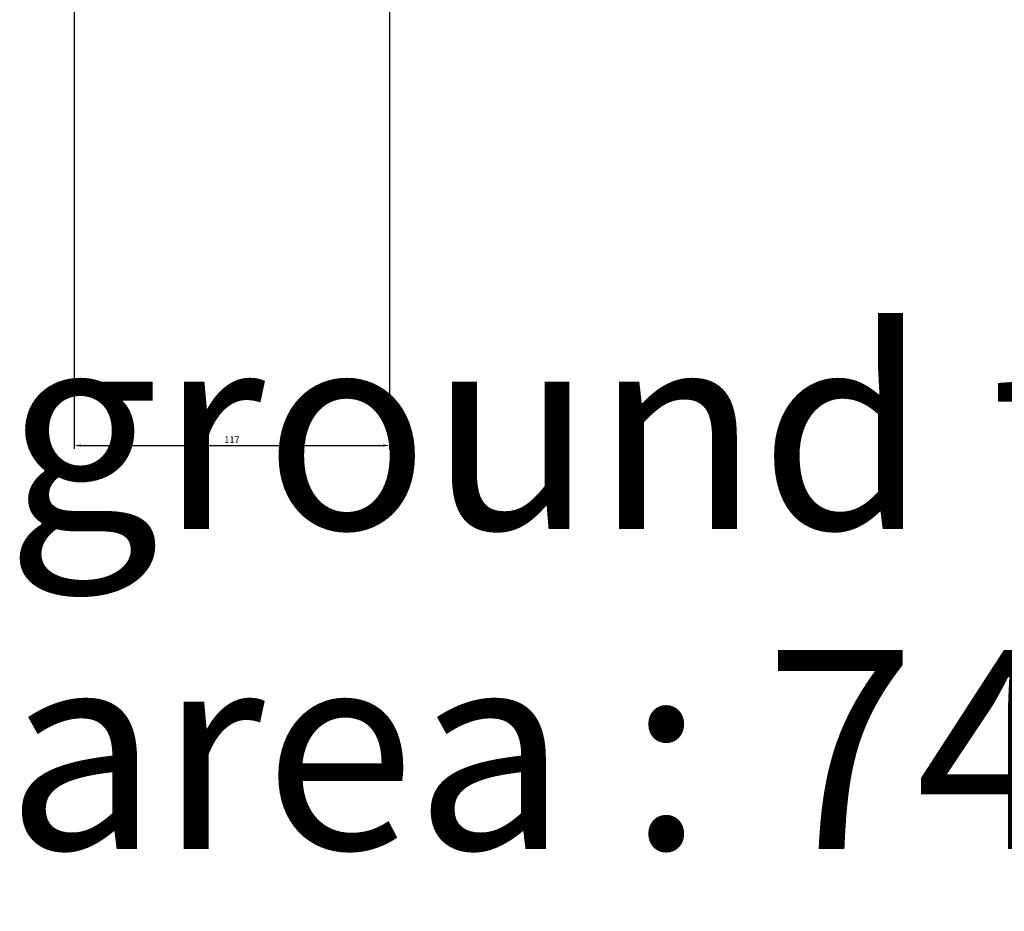
# Model space of a CAD drawing. Units: inches. Extents: x 604 to 3492, y -123 to 1737.
# Tile 1 of 20: x 673 to 1038, y -104 to 227. Entities that reach past the tile are written whole.
import ezdxf

# ---------------------------------------------------------------- set-up
doc = ezdxf.new("R2010")
doc.units = ezdxf.units.IN
for name, color, linetype, lineweight in [('A-ANNO-DIMS', 2, 'Continuous', 18), ('A-ANNO-TEXT', 7, 'Continuous', 35), ('A-AREA-IDEN', 7, 'Continuous', 25)]:
    doc.layers.add(name, color=color, linetype=linetype, lineweight=lineweight)
doc.styles.get("Standard").update_dxf_attribs({"font": 'arial.ttf'})
doc.dimstyles.new('ISO-25', dxfattribs={"dimtxt": 2.5, "dimasz": 2.5, "dimexe": 1.25, "dimexo": 0.625, "dimtad": 1, "dimtxsty": 'Standard', "dimcen": 2.5, "dimadec": 0, "dimazin": 0, "dimtfac": 1, "dimtmove": 0, "dimatfit": 3, "dimfxl": 1, "dimarcsym": 0})

# ---------------------------------------------------------------- blocks, each defined once
blk = doc.blocks.new('*D85')
at = {"layer": 'A-ANNO-DIMS', "color": 0, "lineweight": -2, "transparency": 16777216}
for p, q in [((693.01, 1272.08), (693.01, 67.77)), ((810.01, 1272.08), (810.01, 67.77)), ((695.51, 69.02), (807.51, 69.02))]:
    blk.add_line(p, q, dxfattribs=at)
at = {"layer": 'A-ANNO-DIMS', "color": 0, "transparency": 16777216}
for points in [[(695.51, 69.44), (695.51, 68.61), (693.01, 69.02)], [(807.51, 69.44), (807.51, 68.61), (810.01, 69.02)]]:
    blk.add_solid(points, dxfattribs=at)
at = {"layer": 'Defpoints', "color": 0, "transparency": 16777216}
for p in [(693.01, 1272.7), (810.01, 1272.7), (810.01, 69.02)]:
    blk.add_point(p, dxfattribs=at)
at = {"layer": 'A-ANNO-DIMS', "color": 0, "transparency": 16777216, "insert": (751.51, 70.9), "char_height": 2.5, "attachment_point": 5}
blk.add_mtext('117', dxfattribs=at)

msp = doc.modelspace()

# ---------------------------------------------------------------- texts
at = {"layer": 'A-ANNO-TEXT'}
msp.add_text('ground floor plan', height=73.861865, dxfattribs=at).set_placement((667.6364, 38.0072))
at = {"layer": 'A-AREA-IDEN'}
msp.add_text('area : 749sqft', height=73.861865, dxfattribs=at).set_placement((667.6364, -80.6454))

# ---------------------------------------------------------------- dimensions: what is measured, and where the dimension line sits
at = {"layer": 'A-ANNO-DIMS'}
dim = msp.add_linear_dim(base=(810.0111, 69.0242), p1=(693.0111, 1272.7004), p2=(810.0111, 1272.7004), dimstyle='ISO-25', override={"dimdec": 0, "dimlfac": 1, "dimrnd": 0, "dimzin": 0, "dimdsep": 46, "dimlunit": 2}, dxfattribs=at)
dim.commit()
dim.dimension.update_dxf_attribs({"geometry": '*D85', "text_midpoint": (751.5111, 70.9043)})

doc.saveas('drawing.dxf')
